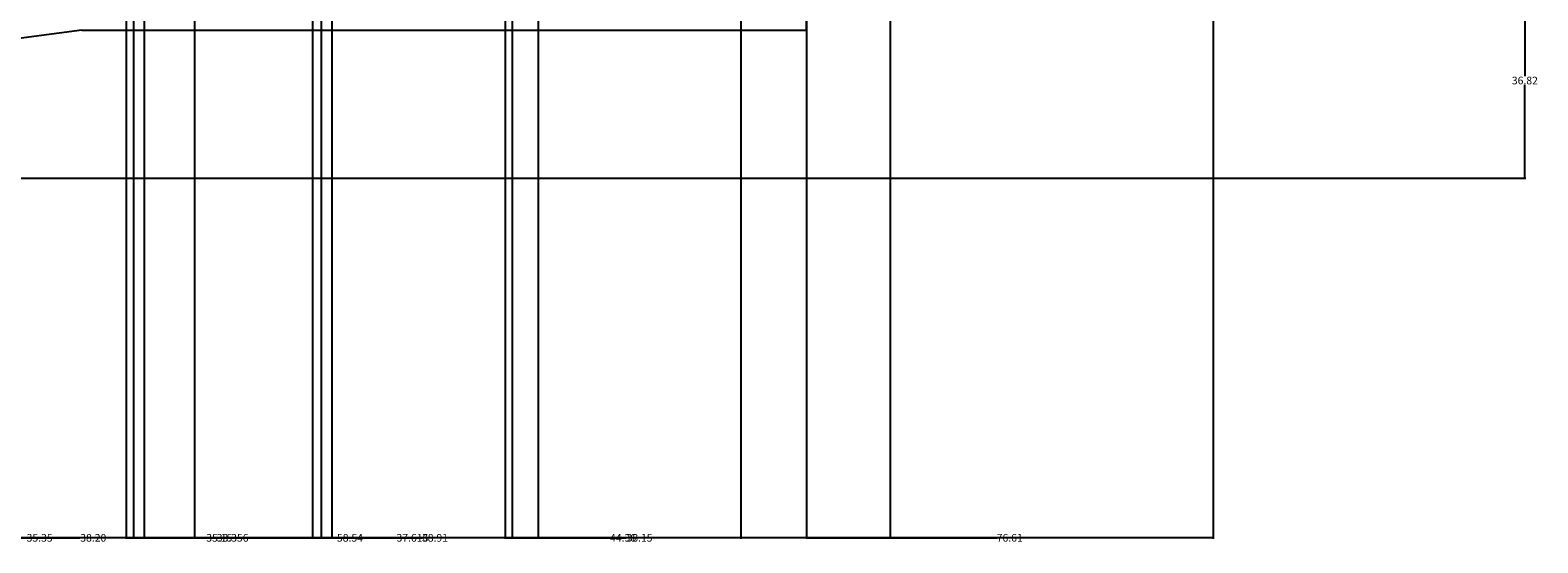
# Model space of a CAD drawing. Units: inches. Extents: x 241 to 943, y 109 to 1396.
# Tile 4 of 34: x 659 to 943, y 109 to 206. Entities that reach past the tile are written whole.
import ezdxf

# ---------------------------------------------------------------- set-up
doc = ezdxf.new("R2010")
doc.units = ezdxf.units.IN
doc.header["$MEASUREMENT"] = 0
doc.layers.add('A-ANNO-DIMS', color=2, linetype='Continuous', lineweight=18)
doc.layers.add('A-ELEV', color=7, linetype='Continuous', lineweight=25)
doc.styles.get("Standard").update_dxf_attribs({"font": 'arial.ttf'})
doc.dimstyles.get("Standard").update_dxf_attribs({"dimtxt": 1.4375, "dimasz": 0.18, "dimexe": 0.18, "dimexo": 0.0625, "dimgap": 0.09, "dimtad": 0, "dimtih": 1, "dimtoh": 1, "dimdec": 4, "dimzin": 0, "dimdsep": 46, "dimlunit": 4, "dimtxsty": 'Standard', "dimcen": 0.09, "dimadec": 0, "dimazin": 0, "dimtfac": 1, "dimtdec": 4, "dimtofl": 0, "dimtmove": 0, "dimatfit": 3, "dimfxl": 1, "dimtolj": 1, "dimtzin": 0, "dimarcsym": 0})

# ---------------------------------------------------------------- blocks, each defined once
blk = doc.blocks.new('*D4')
at = {"layer": 'A-ANNO-DIMS', "color": 0, "lineweight": -2, "transparency": 16777216}
for p, q in [((820.84, 232.77), (820.84, 109.81)), ((377.04, 177.64), (377.04, 109.81)), ((377.22, 109.99), (596.39, 109.99)), ((820.66, 109.99), (601.48, 109.99))]:
    blk.add_line(p, q, dxfattribs=at)
at = {"layer": 'A-ANNO-DIMS', "color": 0, "transparency": 16777216}
for points in [[(377.22, 110.02), (377.22, 109.96), (377.04, 109.99)], [(820.66, 110.02), (820.66, 109.96), (820.84, 109.99)]]:
    blk.add_solid(points, dxfattribs=at)
at = {"layer": 'Defpoints', "color": 0, "transparency": 16777216}
for p in [(820.84, 232.83), (377.04, 177.7), (820.84, 109.99)]:
    blk.add_point(p, dxfattribs=at)
at = {"layer": 'A-ANNO-DIMS', "color": 0, "transparency": 16777216, "insert": (598.94, 109.99), "char_height": 1.438, "attachment_point": 5}
blk.add_mtext('\\A1;443.8', dxfattribs=at)
blk = doc.blocks.new('*D75')
at = {"layer": 'A-ANNO-DIMS', "color": 0, "lineweight": -2, "transparency": 16777216}
for p, q in [((667.46, 214.52), (940.6, 214.52)), ((940.42, 214.34), (940.42, 196.93)), ((940.42, 177.88), (940.42, 195.28)), ((377.1, 177.7), (940.6, 177.7))]:
    blk.add_line(p, q, dxfattribs=at)
at = {"layer": 'A-ANNO-DIMS', "color": 0, "transparency": 16777216}
for points in [[(940.39, 214.34), (940.45, 214.34), (940.42, 214.52)], [(940.39, 177.88), (940.45, 177.88), (940.42, 177.7)]]:
    blk.add_solid(points, dxfattribs=at)
at = {"layer": 'Defpoints', "color": 0, "transparency": 16777216}
for p in [(667.39, 214.52), (940.42, 214.52), (377.04, 177.7)]:
    blk.add_point(p, dxfattribs=at)
at = {"layer": 'A-ANNO-DIMS', "color": 0, "transparency": 16777216, "insert": (940.42, 196.11), "char_height": 1.438, "attachment_point": 5}
blk.add_mtext('\\A1;36.82', dxfattribs=at)
blk = doc.blocks.new('*D77')
at = {"layer": 'A-ANNO-DIMS', "color": 0, "lineweight": -2, "transparency": 16777216}
for p, q in [((805.06, 223.77), (805.06, 109.81)), ((881.67, 223.77), (881.67, 109.81)), ((805.24, 109.99), (840.99, 109.99)), ((881.49, 109.99), (845.73, 109.99))]:
    blk.add_line(p, q, dxfattribs=at)
at = {"layer": 'A-ANNO-DIMS', "color": 0, "transparency": 16777216}
for points in [[(805.24, 110.02), (805.24, 109.96), (805.06, 109.99)], [(881.49, 110.02), (881.49, 109.96), (881.67, 109.99)]]:
    blk.add_solid(points, dxfattribs=at)
at = {"layer": 'Defpoints', "color": 0, "transparency": 16777216}
for p in [(805.06, 223.83), (881.67, 223.83), (881.67, 109.99)]:
    blk.add_point(p, dxfattribs=at)
at = {"layer": 'A-ANNO-DIMS', "color": 0, "transparency": 16777216, "insert": (843.36, 109.99), "char_height": 1.438, "attachment_point": 5}
blk.add_mtext('\\A1;76.61', dxfattribs=at)
blk = doc.blocks.new('*D97')
at = {"layer": 'A-ANNO-DIMS', "color": 0, "lineweight": -2, "transparency": 16777216}
for p, q in [((881.67, 223.77), (881.67, 109.81)), ((303.24, 168.68), (303.24, 109.81)), ((303.42, 109.99), (589.38, 109.99)), ((881.49, 109.99), (595.53, 109.99))]:
    blk.add_line(p, q, dxfattribs=at)
at = {"layer": 'A-ANNO-DIMS', "color": 0, "transparency": 16777216}
for points in [[(303.42, 110.02), (303.42, 109.96), (303.24, 109.99)], [(881.49, 110.02), (881.49, 109.96), (881.67, 109.99)]]:
    blk.add_solid(points, dxfattribs=at)
at = {"layer": 'Defpoints', "color": 0, "transparency": 16777216}
for p in [(881.67, 223.83), (303.24, 168.74), (881.67, 109.99)]:
    blk.add_point(p, dxfattribs=at)
at = {"layer": 'A-ANNO-DIMS', "color": 0, "transparency": 16777216, "insert": (592.45, 109.99), "char_height": 1.438, "attachment_point": 5}
blk.add_mtext('\\A1;578.43', dxfattribs=at)
blk = doc.blocks.new('*D99')
at = {"layer": 'A-ANNO-DIMS', "color": 0, "lineweight": -2, "transparency": 16777216}
for p, q in [((417.09, 181.71), (417.09, 1395.05)), ((417.27, 1394.87), (539.16, 1394.87)), ((667.21, 1394.87), (545.33, 1394.87)), ((667.39, 214.58), (667.39, 1395.05))]:
    blk.add_line(p, q, dxfattribs=at)
at = {"layer": 'A-ANNO-DIMS', "color": 0, "transparency": 16777216}
for points in [[(417.27, 1394.9), (417.27, 1394.84), (417.09, 1394.87)], [(667.21, 1394.9), (667.21, 1394.84), (667.39, 1394.87)]]:
    blk.add_solid(points, dxfattribs=at)
at = {"layer": 'Defpoints', "color": 0, "transparency": 16777216}
for p in [(667.39, 1394.87), (667.39, 214.52), (417.09, 181.65)]:
    blk.add_point(p, dxfattribs=at)
at = {"layer": 'A-ANNO-DIMS', "color": 0, "transparency": 16777216, "insert": (542.24, 1394.87), "char_height": 1.438, "attachment_point": 5}
blk.add_mtext('\\A1;250.30', dxfattribs=at)
blk = doc.blocks.new('*D120')
at = {"layer": 'A-ANNO-DIMS', "color": 0, "lineweight": -2, "transparency": 16777216}
for p, q in [((642.92, 734.79), (642.92, 109.81)), ((678.27, 734.79), (678.27, 109.81)), ((643.1, 109.99), (658.07, 109.99)), ((678.09, 109.99), (663.11, 109.99))]:
    blk.add_line(p, q, dxfattribs=at)
at = {"layer": 'A-ANNO-DIMS', "color": 0, "transparency": 16777216}
for points in [[(643.1, 110.02), (643.1, 109.96), (642.92, 109.99)], [(678.09, 110.02), (678.09, 109.96), (678.27, 109.99)]]:
    blk.add_solid(points, dxfattribs=at)
at = {"layer": 'Defpoints', "color": 0, "transparency": 16777216}
for p in [(642.92, 734.85), (678.27, 734.85), (678.27, 109.99)]:
    blk.add_point(p, dxfattribs=at)
at = {"layer": 'A-ANNO-DIMS', "color": 0, "transparency": 16777216, "insert": (660.59, 109.99), "char_height": 1.438, "attachment_point": 5}
blk.add_mtext('\\A1;35.35', dxfattribs=at)
blk = doc.blocks.new('*D121')
at = {"layer": 'A-ANNO-DIMS', "color": 0, "lineweight": -2, "transparency": 16777216}
for p, q in [((680.27, 736.86), (680.27, 109.81)), ((713.62, 736.86), (713.62, 109.81)), ((680.45, 109.99), (693.87, 109.99)), ((713.44, 109.99), (700.02, 109.99))]:
    blk.add_line(p, q, dxfattribs=at)
at = {"layer": 'A-ANNO-DIMS', "color": 0, "transparency": 16777216}
for points in [[(680.45, 110.02), (680.45, 109.96), (680.27, 109.99)], [(713.44, 110.02), (713.44, 109.96), (713.62, 109.99)]]:
    blk.add_solid(points, dxfattribs=at)
at = {"layer": 'Defpoints', "color": 0, "transparency": 16777216}
for p in [(680.27, 736.92), (713.62, 736.92), (713.62, 109.99)]:
    blk.add_point(p, dxfattribs=at)
at = {"layer": 'A-ANNO-DIMS', "color": 0, "transparency": 16777216, "insert": (696.95, 109.99), "char_height": 1.438, "attachment_point": 5}
blk.add_mtext('\\A1;33.356', dxfattribs=at)
blk = doc.blocks.new('*D122')
at = {"layer": 'A-ANNO-DIMS', "color": 0, "lineweight": -2, "transparency": 16777216}
for p, q in [((715.62, 734.79), (715.62, 109.81)), ((754.54, 734.79), (754.54, 109.81)), ((715.8, 109.99), (732.7, 109.99)), ((754.36, 109.99), (737.46, 109.99))]:
    blk.add_line(p, q, dxfattribs=at)
at = {"layer": 'A-ANNO-DIMS', "color": 0, "transparency": 16777216}
for points in [[(715.8, 110.02), (715.8, 109.96), (715.62, 109.99)], [(754.36, 110.02), (754.36, 109.96), (754.54, 109.99)]]:
    blk.add_solid(points, dxfattribs=at)
at = {"layer": 'Defpoints', "color": 0, "transparency": 16777216}
for p in [(715.62, 734.85), (754.54, 734.85), (754.54, 109.99)]:
    blk.add_point(p, dxfattribs=at)
at = {"layer": 'A-ANNO-DIMS', "color": 0, "transparency": 16777216, "insert": (735.08, 109.99), "char_height": 1.438, "attachment_point": 5}
blk.add_mtext('\\A1;38.91', dxfattribs=at)
blk = doc.blocks.new('*D123')
at = {"layer": 'A-ANNO-DIMS', "color": 0, "lineweight": -2, "transparency": 16777216}
for p, q in [((754.54, 734.79), (754.54, 109.81)), ((792.69, 734.79), (792.69, 109.81)), ((754.72, 109.99), (771.09, 109.99)), ((792.51, 109.99), (776.13, 109.99))]:
    blk.add_line(p, q, dxfattribs=at)
at = {"layer": 'A-ANNO-DIMS', "color": 0, "transparency": 16777216}
for points in [[(754.72, 110.02), (754.72, 109.96), (754.54, 109.99)], [(792.51, 110.02), (792.51, 109.96), (792.69, 109.99)]]:
    blk.add_solid(points, dxfattribs=at)
at = {"layer": 'Defpoints', "color": 0, "transparency": 16777216}
for p in [(754.54, 734.85), (792.69, 734.85), (792.69, 109.99)]:
    blk.add_point(p, dxfattribs=at)
at = {"layer": 'A-ANNO-DIMS', "color": 0, "transparency": 16777216, "insert": (773.61, 109.99), "char_height": 1.438, "attachment_point": 5}
blk.add_mtext('\\A1;38.15', dxfattribs=at)
blk = doc.blocks.new('*D132')
at = {"layer": 'A-ANNO-DIMS', "color": 0, "lineweight": -2, "transparency": 16777216}
for p, q in [((676.87, 628.34), (676.87, 109.81)), ((617.76, 626.34), (617.76, 109.81)), ((617.94, 109.99), (644.94, 109.99)), ((676.69, 109.99), (649.69, 109.99))]:
    blk.add_line(p, q, dxfattribs=at)
at = {"layer": 'A-ANNO-DIMS', "color": 0, "transparency": 16777216}
for points in [[(617.94, 110.02), (617.94, 109.96), (617.76, 109.99)], [(676.69, 110.02), (676.69, 109.96), (676.87, 109.99)]]:
    blk.add_solid(points, dxfattribs=at)
at = {"layer": 'Defpoints', "color": 0, "transparency": 16777216}
for p in [(676.87, 628.4), (617.76, 626.4), (676.87, 109.99)]:
    blk.add_point(p, dxfattribs=at)
at = {"layer": 'A-ANNO-DIMS', "color": 0, "transparency": 16777216, "insert": (647.31, 109.99), "char_height": 1.438, "attachment_point": 5}
blk.add_mtext('\\A1;59.11', dxfattribs=at)
blk = doc.blocks.new('*D133')
at = {"layer": 'A-ANNO-DIMS', "color": 0, "lineweight": -2, "transparency": 16777216}
for p, q in [((676.87, 628.34), (676.87, 109.81)), ((712.02, 628.34), (712.02, 109.81)), ((677.05, 109.99), (691.92, 109.99)), ((711.84, 109.99), (696.96, 109.99))]:
    blk.add_line(p, q, dxfattribs=at)
at = {"layer": 'A-ANNO-DIMS', "color": 0, "transparency": 16777216}
for points in [[(677.05, 110.02), (677.05, 109.96), (676.87, 109.99)], [(711.84, 110.02), (711.84, 109.96), (712.02, 109.99)]]:
    blk.add_solid(points, dxfattribs=at)
at = {"layer": 'Defpoints', "color": 0, "transparency": 16777216}
for p in [(676.87, 628.4), (712.02, 628.4), (712.02, 109.99)]:
    blk.add_point(p, dxfattribs=at)
at = {"layer": 'A-ANNO-DIMS', "color": 0, "transparency": 16777216, "insert": (694.44, 109.99), "char_height": 1.438, "attachment_point": 5}
blk.add_mtext('\\A1;35.15', dxfattribs=at)
blk = doc.blocks.new('*D134')
at = {"layer": 'A-ANNO-DIMS', "color": 0, "lineweight": -2, "transparency": 16777216}
for p, q in [((712.02, 628.34), (712.02, 109.81)), ((749.63, 626.34), (749.63, 109.81)), ((712.2, 109.99), (727.75, 109.99)), ((749.45, 109.99), (733.9, 109.99))]:
    blk.add_line(p, q, dxfattribs=at)
at = {"layer": 'A-ANNO-DIMS', "color": 0, "transparency": 16777216}
for points in [[(712.2, 110.02), (712.2, 109.96), (712.02, 109.99)], [(749.45, 110.02), (749.45, 109.96), (749.63, 109.99)]]:
    blk.add_solid(points, dxfattribs=at)
at = {"layer": 'Defpoints', "color": 0, "transparency": 16777216}
for p in [(712.02, 628.4), (749.63, 626.4), (749.63, 109.99)]:
    blk.add_point(p, dxfattribs=at)
at = {"layer": 'A-ANNO-DIMS', "color": 0, "transparency": 16777216, "insert": (730.82, 109.99), "char_height": 1.438, "attachment_point": 5}
blk.add_mtext('\\A1;37.616', dxfattribs=at)
blk = doc.blocks.new('*D142')
at = {"layer": 'A-ANNO-DIMS', "color": 0, "lineweight": -2, "transparency": 16777216}
for p, q in [((689.79, 498.38), (689.79, 109.81)), ((651.6, 496.38), (651.6, 109.81)), ((651.78, 109.99), (668.18, 109.99)), ((689.61, 109.99), (673.21, 109.99))]:
    blk.add_line(p, q, dxfattribs=at)
at = {"layer": 'A-ANNO-DIMS', "color": 0, "transparency": 16777216}
for points in [[(651.78, 110.02), (651.78, 109.96), (651.6, 109.99)], [(689.61, 110.02), (689.61, 109.96), (689.79, 109.99)]]:
    blk.add_solid(points, dxfattribs=at)
at = {"layer": 'Defpoints', "color": 0, "transparency": 16777216}
for p in [(689.79, 498.44), (651.6, 496.44), (689.79, 109.99)]:
    blk.add_point(p, dxfattribs=at)
at = {"layer": 'A-ANNO-DIMS', "color": 0, "transparency": 16777216, "insert": (670.7, 109.99), "char_height": 1.438, "attachment_point": 5}
blk.add_mtext('\\A1;38.20', dxfattribs=at)
blk = doc.blocks.new('*D143')
at = {"layer": 'A-ANNO-DIMS', "color": 0, "lineweight": -2, "transparency": 16777216}
for p, q in [((689.79, 498.38), (689.79, 109.81)), ((748.33, 498.38), (748.33, 109.81)), ((689.97, 109.99), (716.55, 109.99)), ((748.15, 109.99), (721.58, 109.99))]:
    blk.add_line(p, q, dxfattribs=at)
at = {"layer": 'A-ANNO-DIMS', "color": 0, "transparency": 16777216}
for points in [[(689.97, 110.02), (689.97, 109.96), (689.79, 109.99)], [(748.15, 110.02), (748.15, 109.96), (748.33, 109.99)]]:
    blk.add_solid(points, dxfattribs=at)
at = {"layer": 'Defpoints', "color": 0, "transparency": 16777216}
for p in [(689.79, 498.44), (748.33, 498.44), (748.33, 109.99)]:
    blk.add_point(p, dxfattribs=at)
at = {"layer": 'A-ANNO-DIMS', "color": 0, "transparency": 16777216, "insert": (719.06, 109.99), "char_height": 1.438, "attachment_point": 5}
blk.add_mtext('\\A1;58.54', dxfattribs=at)
blk = doc.blocks.new('*D144')
at = {"layer": 'A-ANNO-DIMS', "color": 0, "lineweight": -2, "transparency": 16777216}
for p, q in [((748.33, 498.38), (748.33, 109.81)), ((792.69, 496.38), (792.69, 109.81)), ((748.51, 109.99), (767.97, 109.99)), ((792.51, 109.99), (773.06, 109.99))]:
    blk.add_line(p, q, dxfattribs=at)
at = {"layer": 'A-ANNO-DIMS', "color": 0, "transparency": 16777216}
for points in [[(748.51, 110.02), (748.51, 109.96), (748.33, 109.99)], [(792.51, 110.02), (792.51, 109.96), (792.69, 109.99)]]:
    blk.add_solid(points, dxfattribs=at)
at = {"layer": 'Defpoints', "color": 0, "transparency": 16777216}
for p in [(748.33, 498.44), (792.69, 496.44), (792.69, 109.99)]:
    blk.add_point(p, dxfattribs=at)
at = {"layer": 'A-ANNO-DIMS', "color": 0, "transparency": 16777216, "insert": (770.51, 109.99), "char_height": 1.438, "attachment_point": 5}
blk.add_mtext('\\A1;44.36', dxfattribs=at)

msp = doc.modelspace()

# ---------------------------------------------------------------- linework, layer by layer
at = {"layer": 'A-ELEV'}
for p, q in [((805.0568, 205.5955), (805.0568, 223.8295)), ((668.5653, 205.5955), (418.2631, 172.7256)), ((668.5653, 205.5955), (796.0568, 205.5955)), ((796.0568, 205.5955), (805.0568, 205.5955))]:
    msp.add_line(p, q, dxfattribs=at)

# ---------------------------------------------------------------- dimensions: what is measured, and where the dimension line sits
at = {"layer": 'A-ANNO-DIMS'}
for base, p1, p2, override, picture, middle in [((667.3935, 1394.8654), (417.0913, 181.649), (667.3935, 214.5189), {"dimdec": 2, "dimlfac": 1, "dimrnd": 0, "dimzin": 0, "dimdsep": 46, "dimlunit": 2}, '*D99', (542.2424, 1394.8654)), ((713.6236, 109.9907), (680.2674, 736.9235), (713.6236, 736.9235), {"dimdec": 3, "dimlfac": 1, "dimrnd": 0, "dimzin": 0, "dimdsep": 46, "dimlunit": 2}, '*D121', (696.9455, 109.9907)), ((678.2674, 109.9907), (642.9197, 734.8538), (678.2674, 734.8538), {"dimdec": 2, "dimlfac": 1, "dimrnd": 0, "dimzin": 0, "dimdsep": 46, "dimlunit": 2}, '*D120', (660.5935, 109.9907)), ((754.5373, 109.9907), (715.6236, 734.8538), (754.5373, 734.8538), {"dimdec": 2, "dimlfac": 1, "dimrnd": 0, "dimzin": 0, "dimdsep": 46, "dimlunit": 2}, '*D122', (735.0804, 109.9907)), ((792.691, 109.9907), (754.5373, 734.8538), (792.691, 734.8538), {"dimdec": 2, "dimlfac": 1, "dimrnd": 0, "dimzin": 0, "dimdsep": 46, "dimlunit": 2}, '*D123', (773.6142, 109.9907)), ((676.8698, 109.9907), (617.7594, 626.4013), (676.8698, 628.4013), {"dimdec": 2, "dimlfac": 1, "dimrnd": 0, "dimzin": 0, "dimdsep": 46, "dimlunit": 2}, '*D132', (647.3146, 109.9907)), ((712.0171, 109.9907), (676.8698, 628.4013), (712.0171, 628.4013), {"dimdec": 2, "dimlfac": 1, "dimrnd": 0, "dimzin": 0, "dimdsep": 46, "dimlunit": 2}, '*D133', (694.4435, 109.9907)), ((749.6328, 109.9907), (712.0171, 628.4013), (749.6328, 626.4013), {"dimdec": 3, "dimlfac": 1, "dimrnd": 0, "dimzin": 0, "dimdsep": 46, "dimlunit": 2}, '*D134', (730.825, 109.9907)), ((689.794, 109.9907), (651.5974, 496.4395), (689.794, 498.4395), {"dimdec": 2, "dimlfac": 1, "dimrnd": 0, "dimzin": 0, "dimdsep": 46, "dimlunit": 2}, '*D142', (670.6957, 109.9907)), ((748.3325, 109.9907), (689.794, 498.4395), (748.3325, 498.4395), {"dimdec": 2, "dimlfac": 1, "dimrnd": 0, "dimzin": 0, "dimdsep": 46, "dimlunit": 2}, '*D143', (719.0633, 109.9907)), ((792.691, 109.9907), (748.3325, 498.4395), (792.691, 496.4395), {"dimdec": 2, "dimlfac": 1, "dimrnd": 0, "dimzin": 0, "dimdsep": 46, "dimlunit": 2}, '*D144', (770.5118, 109.9907)), ((820.8374, 109.9907), (377.0391, 177.6977), (820.8374, 232.8295), {"dimdec": 1, "dimlfac": 1, "dimrnd": 0, "dimzin": 0, "dimdsep": 46, "dimlunit": 2}, '*D4', (598.9383, 109.9907)), ((881.667, 109.9907), (303.2358, 168.7407), (881.667, 223.8295), {"dimdec": 2, "dimlfac": 1, "dimrnd": 0, "dimzin": 0, "dimdsep": 46, "dimlunit": 2}, '*D97', (592.4514, 109.9907)), ((881.667, 109.9907), (805.0568, 223.8295), (881.667, 223.8295), {"dimdec": 2, "dimlfac": 1, "dimrnd": 0, "dimzin": 0, "dimdsep": 46, "dimlunit": 2}, '*D77', (843.3619, 109.9907))]:
    dim = msp.add_linear_dim(base=base, p1=p1, p2=p2, dimstyle='Standard', override=override, dxfattribs=at)
    dim.commit()
    dim.dimension.update_dxf_attribs({"geometry": picture, "text_midpoint": middle})
dim = msp.add_linear_dim(base=(940.417, 214.5189), p1=(377.0391, 177.6977), p2=(667.3935, 214.5189), angle=90, dimstyle='Standard', override={"dimdec": 2, "dimlfac": 1, "dimrnd": 0, "dimzin": 0, "dimdsep": 46, "dimlunit": 2}, dxfattribs=at)
dim.commit()
dim.dimension.update_dxf_attribs({"geometry": '*D75', "text_midpoint": (940.417, 196.1083)})

doc.saveas('drawing.dxf')
